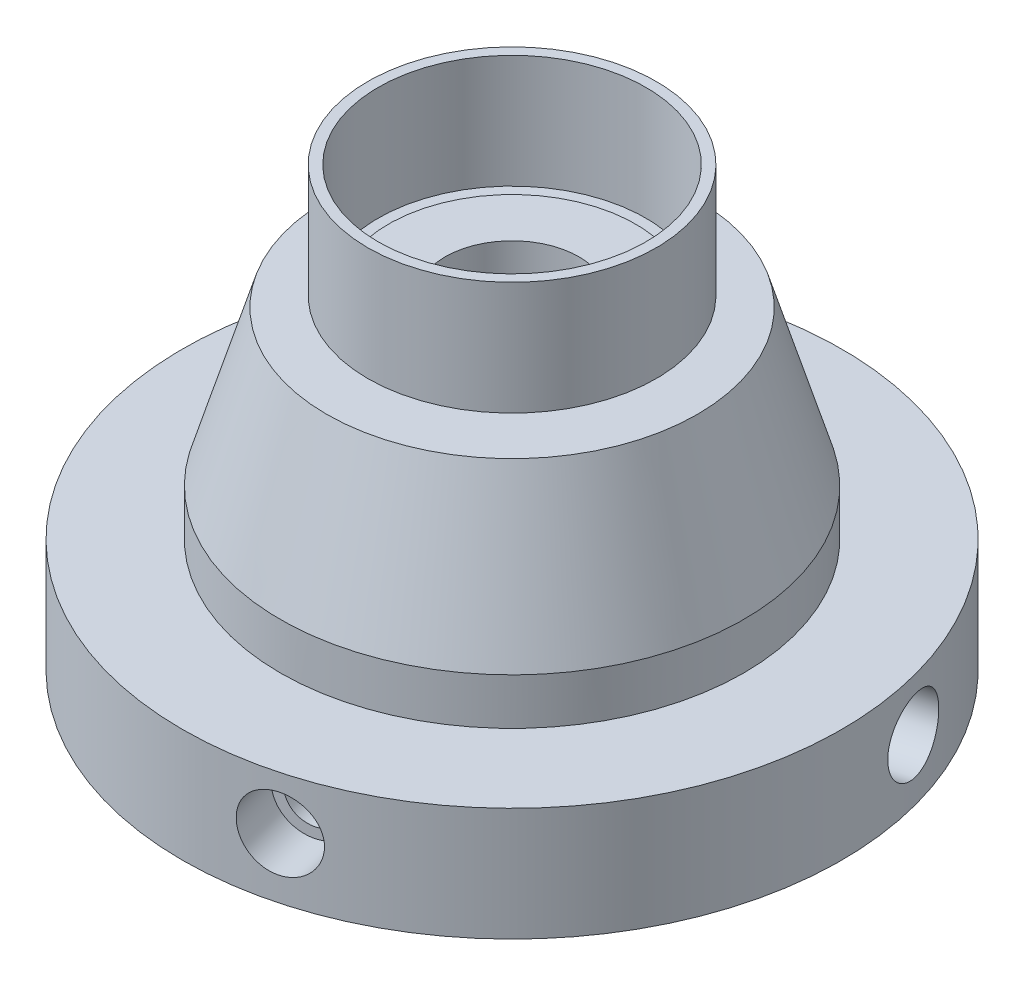
SolidWorks part; units mm, degrees
material "Plain Carbon Steel"
ref_plane "Front Plane" through (0, 0, 0) normal (0, 0, 1) x (1, 0, 0)
ref_plane "Top Plane" through (0, 0, 0) normal (0, 1, 0) x (1, 0, 0)
ref_plane "Right Plane" through (0, 0, 0) normal (1, 0, 0) x (0, 0, -1)
sketch "Base Flange Sketch" plane through (0, 0, 0) normal (0, 1, 0) x (1, 0, 0)
  line L0 (0, 80.3022) -> (0, -67.8029) construction
  line L1 (139.8508, 0) -> (-140.0866, 0) construction
  circle A0 centre (0, 0) radius 64
  dimension "D1" = 128
extrude "Base Flange Ø128" add sketch "Base Flange Sketch" along normal blind 22
sketch "Collar Sketch" plane through (0, 22, 0) normal (0, 1, 0) x (1, 0, 0)
  circle A0 centre (0, 0) radius 45
  dimension "D1" = 90
extrude "Collar Ø90" add sketch "Collar Sketch" along normal blind 9 contours A0
ref_plane "Loft Top Plane" through (0, 61, 0) normal (0, 1, 0) x (1, 0, 0)
sketch "Loft Top Profile Ø72" plane through (0, 61, 0) normal (0, 1, 0) x (1, 0, 0)
  circle A0 centre (0, 0) radius 36
  dimension "D1" = 72
sketch "Loft Base Profile" plane through (0, 31, 0) normal (0, 1, 0) x (1, 0, 0)
  circle A0 centre (0, 0) radius 45 construction
  circle A1 centre (0, 0) radius 45
loft "Conical Transition Loft" add profiles "Loft Base Profile", "Loft Top Profile Ø72"
sketch "Sketch6" plane through (0, 61, 0) normal (0, 1, 0) x (1, 0, 0)
  circle A0 centre (0, 0) radius 28
  dimension "D1" = 56
sketch "Top Step Sketch" plane through (0, 61, 0) normal (0, 1, 0) x (1, 0, 0)
  circle A1 centre (0, 0) radius 24
  dimension "D2" = 48
extrude "Top Step Ø48" add sketch "Top Step Sketch" along normal blind 2 contours A1
sketch "Tube Sketch" plane through (0, 63, 0) normal (0, 1, 0) x (1, 0, 0)
  circle A0 centre (0, 0) radius 26
  circle A1 centre (0, 0) radius 28
  dimension "D1" = 52
  dimension "D2" = 56
extrude "Tube Ø56xØ52" add sketch "Tube Sketch" along normal blind 22 separate body
hole_wizard "Radial C-Bore Hole Ø10" positions "3DSketch2" profile "Sketch15" legacy
sketch3d "3DSketch2"
  point P0 (61.8225, 11.6871, -16.5523)
sketch "Sketch15" plane through (61.8225, 11.6871, -16.5523) normal (0, 1, 0) x (-0.2586, 0, -0.966)
  line L0 (0, 0) -> (0, 45)
  line L1 (0, 45) -> (5, 45)
  line L2 (5, 45) -> (5, 10)
  line L3 (5, 10) -> (7, 10)
  line L4 (7, 10) -> (7, 0)
  line L5 (7, 0) -> (0, 0)
  line L6 (0, 110) -> (0, -10) construction
  dimension "Diameter" = 10
  dimension "Depth" = 45
  dimension "C-Bore Diameter" = 14
  dimension "C-Bore Depth" = 10
pattern_circular "Radial Holes Pattern 4x" count 4 over 360 about axis through (0, 0, 0) along (0, 1, 0) of "Radial C-Bore Hole Ø10"
sketch "Bottom Recess Sketch" plane through (0, 0, 0) normal (0, -1, 0) x (1, 0, 0)
  circle A0 centre (0, 0) radius 31
  dimension "D1" = 62
extrude "Bottom Recess Ø62" cut sketch "Bottom Recess Sketch" against normal blind 6
sketch "Bottom Slot Sketch" plane through (0, 6, 0) normal (0, -1, 0) x (1, 0, 0)
  line L1 (12.7574, 2.5) -> (16, 2.5)
  line L3 (12.7574, -2.5) -> (16, -2.5)
  line L4 (16, 2.5) -> (16, -2.5)
  arc A0 (12.7574, 2.5) -> (12.7574, -2.5) centre (0, 0) ccw
  circle A2 centre (0, 0) radius 31 construction
  dimension "D1" = 26
  dimension "D2" = 5
  dimension "D3" = 16
extrude "Bottom Slot Cut" cut sketch "Bottom Slot Sketch" against normal up to next (57 mm away)
